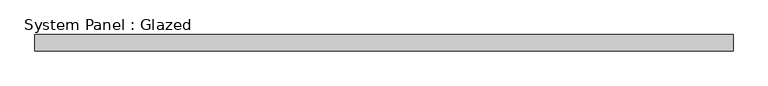
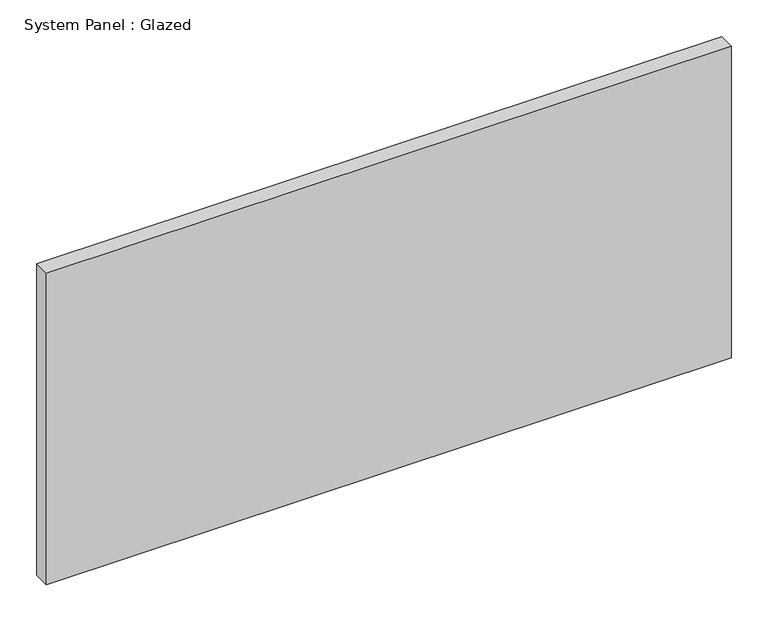
"""IFC4 building model written with IfcOpenShell, lengths in millimetres: plate geometry, System Panel : Glazed."""

from ifc_helpers import new_model, si_unit, origin, origin_with_axes, place, context, project, spatial, polyline, outline, extrude, source, transform, mapped, element, save


def system_panel_glazed_03e0ee66(model_context):
    return source(origin(), model_context, "Body", "SweptSolid", [
        extrude(outline(polyline([(534.4583334, 19.05), (-534.4583334, 19.05), (-534.4583334, 44.45), (534.4583334, 44.45), (534.4583334, 19.05)])), origin_with_axes(), (0.0, 0.0, 1.0), 514.35),
    ])


if __name__ == "__main__":
    model = new_model("IFC4")
    model_context = context("Model", 3, world=origin())
    ifc_project = project(units=[si_unit("LENGTHUNIT", "METRE", prefix="MILLI")], contexts=[model_context])
    site = spatial("IfcSite", under=ifc_project)
    building = spatial("IfcBuilding", under=site)
    placement = place(None, origin())
    system_panel_glazed_shape = system_panel_glazed_03e0ee66(model_context)
    element("IfcPlate", 1, ObjectType="System Panel : Glazed", at=placement, inside=building, context=model_context, shape_type="MappedRepresentation", body=[
        mapped(system_panel_glazed_shape, transform((0.0, 0.0, 0.0), x_axis=(1.0, 0.0, 0.0), y_axis=(0.0, 1.0, 0.0), z_axis=(0.0, 0.0, 1.0))),
    ])
    save(model, "model.ifc")

# Revit data of these elements
# Type "System Panel : Glazed"
#   Construction Type Id = "GSP4R"
#   Analytic Construction = "1/8 in Pilkington single glazing"
#   Visual Light Transmittance = 0.9
#   Solar Heat Gain Coefficient = 0.86
#   Heat Transfer Coefficient (U) = 1.18115 BTU/(h·ft²·°F)
#   Define Thermal Properties by = 1
# Element 1 (IfcPlate, "System Panel : Glazed")
#   Materials on its faces: "Glass"
# Materials
#   "Glass": class "Glass", colour RGB 0 128 192, transparency 0.75, Description = "Soda Lime Glass", Cost = 0
